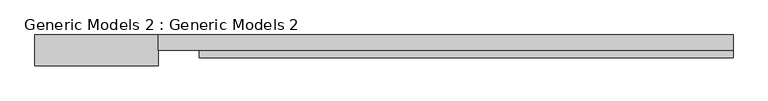
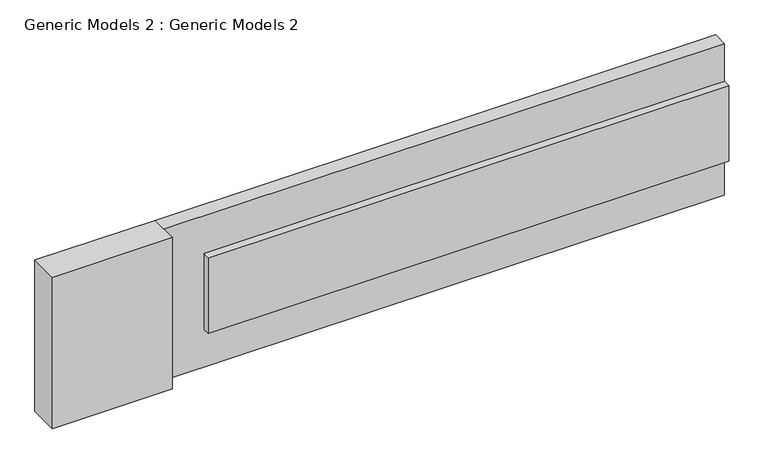
"""IFC4 building model written with IfcOpenShell, lengths in millimetres: proxy geometry, Generic Models 2 : Generic Models 2."""

from ifc_helpers import new_model, si_unit, frame, origin, place, context, project, spatial, polyline, outline, extrude, source, transform, mapped, element, save


def generic_models_2_generic_models_2_f62d3e83(model_context):
    return source(origin(), model_context, "Body", "SweptSolid", [
        extrude(outline(polyline([(-8511.7167709, -5862.7399866), (-12474.1167709, -5862.7399866), (-12474.1167709, -5805.8637867), (-8511.7167709, -5805.8637867), (-8511.7167709, -5862.7399866)])), frame((0.0, 0.0, 609.6), z_axis=(0.0, 0.0, 1.0), x_axis=(1.0, 0.0, 0.0)), (0.0, 0.0, 1.0), 609.6),
        extrude(outline(polyline([(-8511.7167709, -5805.8637867), (-12778.9167709, -5805.8637867), (-12778.9167709, -5691.5637867), (-8511.7167709, -5691.5637867), (-8511.7167709, -5805.8637867)])), frame((0.0, 0.0, 304.8), z_axis=(0.0, 0.0, 1.0), x_axis=(1.0, 0.0, 0.0)), (0.0, 0.0, 1.0), 1219.2),
        extrude(outline(polyline([(-12778.9167709, -5920.1637867), (-13693.3167709, -5920.1637867), (-13693.3167709, -5691.5637867), (-12778.9167709, -5691.5637867), (-12778.9167709, -5920.1637867)])), frame((0.0, 0.0, 304.8), z_axis=(0.0, 0.0, 1.0), x_axis=(1.0, 0.0, 0.0)), (0.0, 0.0, 1.0), 1219.2),
    ])


if __name__ == "__main__":
    model = new_model("IFC4")
    model_context = context("Model", 3, world=origin())
    ifc_project = project(units=[si_unit("LENGTHUNIT", "METRE", prefix="MILLI")], contexts=[model_context])
    site = spatial("IfcSite", under=ifc_project)
    building = spatial("IfcBuilding", under=site)
    placement = place(None, origin())
    generic_models_2_generic_models_2_shape = generic_models_2_generic_models_2_f62d3e83(model_context)
    element("IfcBuildingElementProxy", 1, Name="Generic Models 2 : Generic Models 2", ObjectType="Generic Models 2 : Generic Models 2", at=placement, inside=building, context=model_context, shape_type="MappedRepresentation", body=[
        mapped(generic_models_2_generic_models_2_shape, transform((0.0, 0.0, 0.0), x_axis=(1.0, 0.0, 0.0), y_axis=(0.0, 1.0, 0.0), z_axis=(0.0, 0.0, 1.0))),
    ])
    save(model, "model.ifc")
